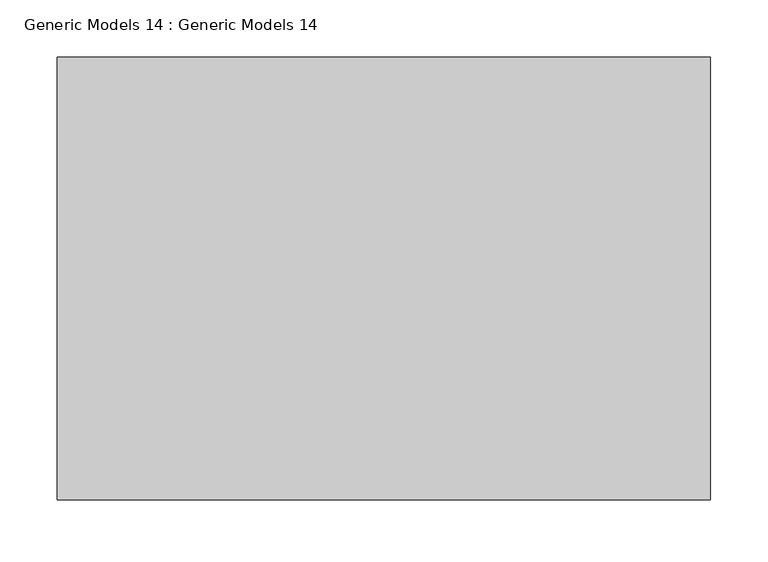
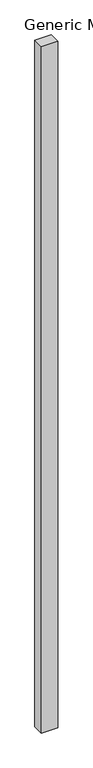
"""IFC4 building model written with IfcOpenShell, lengths in millimetres: proxy geometry, Generic Models 14 : Generic Models 14."""

from ifc_helpers import new_model, si_unit, frame, origin, place, context, project, spatial, polyline, outline, extrude, source, transform, mapped, element, save


def generic_models_14_generic_models_14_86cac6df(model_context):
    return source(origin(), model_context, "Body", "SweptSolid", [
        extrude(outline(polyline([(-501.9629849, -4102.404821), (-501.9629849, -4491.2134113), (-1075.5628101, -4491.2134113), (-1075.5628101, -4102.404821), (-501.9629849, -4102.404821)])), frame((0.0, 0.0, 3576.4988811), z_axis=(0.0, 0.0, 1.0), x_axis=(1.0, 0.0, 0.0)), (0.0, 0.0, 1.0), 25100.4362421),
    ])


if __name__ == "__main__":
    model = new_model("IFC4")
    model_context = context("Model", 3, world=origin())
    ifc_project = project(units=[si_unit("LENGTHUNIT", "METRE", prefix="MILLI")], contexts=[model_context])
    site = spatial("IfcSite", under=ifc_project)
    building = spatial("IfcBuilding", under=site)
    placement = place(None, origin())
    generic_models_14_generic_models_14_shape = generic_models_14_generic_models_14_86cac6df(model_context)
    element("IfcBuildingElementProxy", 1, Name="Generic Models 14 : Generic Models 14", ObjectType="Generic Models 14 : Generic Models 14", at=placement, inside=building, context=model_context, shape_type="MappedRepresentation", body=[
        mapped(generic_models_14_generic_models_14_shape, transform((0.0, 0.0, 0.0), x_axis=(1.0, 0.0, 0.0), y_axis=(0.0, 1.0, 0.0), z_axis=(0.0, 0.0, 1.0))),
    ])
    save(model, "model.ifc")
